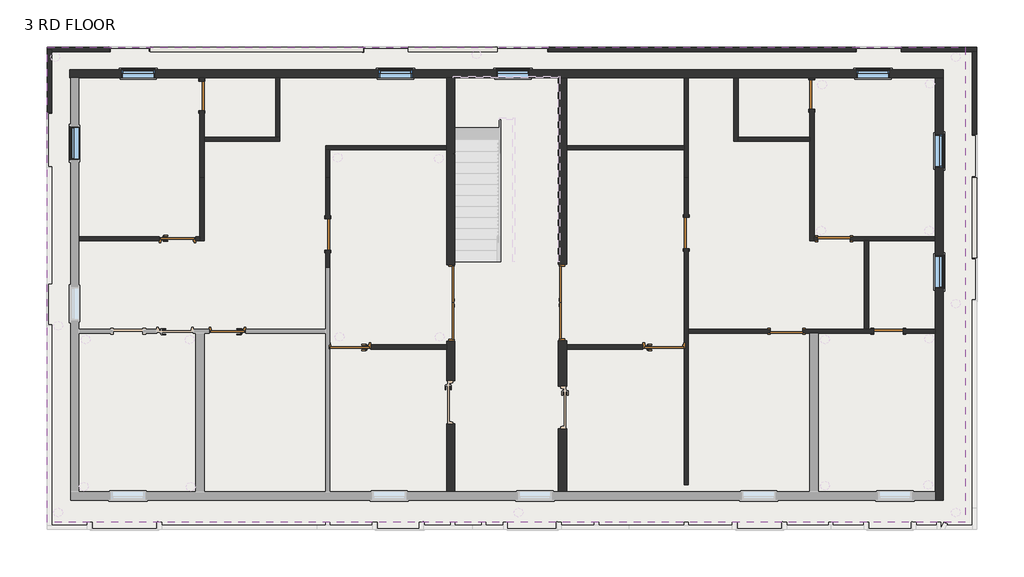
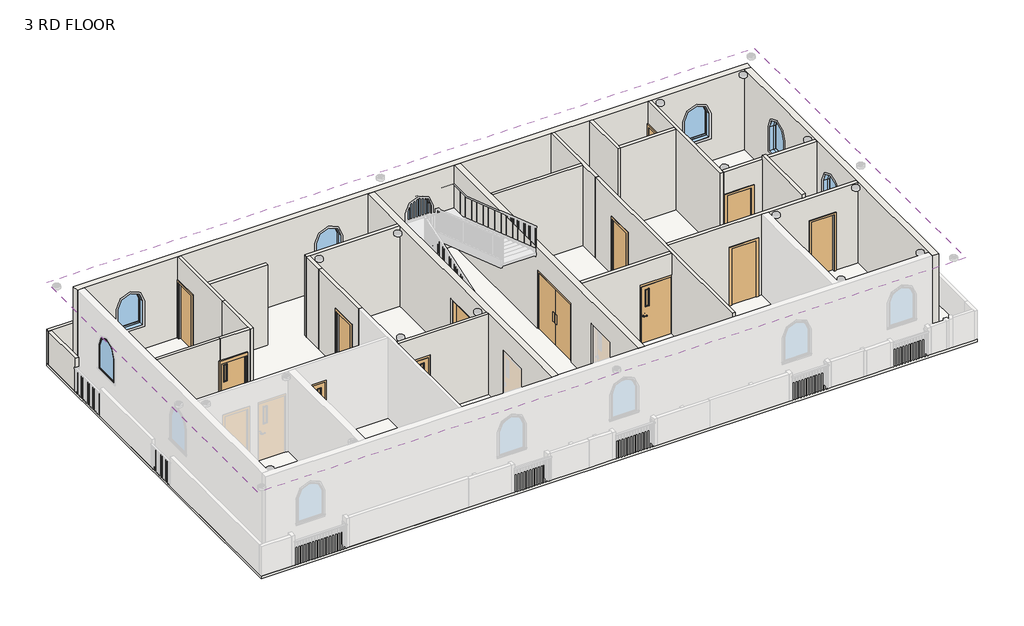
# One storey, part 2 of 7: 33 walls, 13 doors, 7 windows, 1 covering, 1 slab.
"""IFC4 building model written with IfcOpenShell, lengths in millimetres."""

from ifc_helpers import new_model, si_unit, frame, origin, place, context, project, spatial, polyline, circle_curve, outline, extrude, faceted_brep, transform, mapped, element, save
from ifc_brep_helpers import plane_surface, revolved_surface, advanced_brep
from components import door_2c854dd0, door_cf1f2706, door_4f5842df, door_passage_single_vision_lite_3_x7_440dd290, door_70e57c00, door_700d3439, door_8cb1b8a7, door_38851409, door_d141acb4, window_fixed_round_top_3_x_4_dee2be1c

model = new_model("IFC4")

# Units and contexts
model_context = context("Model", 3, world=origin())
ifc_project = project(units=[si_unit("LENGTHUNIT", "METRE", prefix="MILLI")], contexts=[model_context])

# Site, building, storey
site = spatial("IfcSite", under=ifc_project)
building = spatial("IfcBuilding", under=site)
storey = spatial("IfcBuildingStorey", under=building, Name="3 RD FLOOR", Elevation=9601.2)

# Covering
placement = place(None, origin())
element("IfcCovering", 1, ObjectType="2' x 4' ACT System", at=placement, inside=storey, context=model_context, shape_type="SweptSolid", body=[
    extrude(outline(polyline([(12235.5012075, 8470.0067329), (12235.5012075, -4623.6932193), (-13088.8067989, -4623.6932193), (-13088.8067989, 8470.0067329), (12235.5012075, 8470.0067329)])), frame((0.0, 0.0, 12649.2), z_axis=(0.0, 0.0, 1.0), x_axis=(1.0, 0.0, 0.0)), (0.0, 0.0, 1.0), 57.15),
])

# Doors
door_shape = door_2c854dd0(model_context)
element("IfcDoor", 2, ObjectType="Door-Passage-Double-Flush-Dbl_Acting : 6'79\" X 84\"", at=placement, inside=storey, context=model_context, shape_type="MappedRepresentation", body=[
    mapped(door_shape, transform((-1969.4487998, 1424.4578621, 9601.2), x_axis=(0.0, -1.0, 0.0), y_axis=(1.0, 0.0, 0.0), z_axis=(0.0, 0.0, 1.0))),
])
element("IfcDoor", 3, ObjectType="Door-Passage-Double-Flush-Dbl_Acting : 6'79\" X 84\"", at=placement, inside=storey, context=model_context, shape_type="MappedRepresentation", body=[
    mapped(door_shape, transform((1128.8432011, 1434.2067807, 9601.2), x_axis=(0.0, 1.0, 0.0), y_axis=(-1.0, 0.0, 0.0), z_axis=(0.0, 0.0, 1.0))),
])
door_2_shape = door_cf1f2706(model_context)
element("IfcDoor", 4, ObjectType="Door-Passage-Single-Vision_Lite : 3'6\"X7' 2", at=placement, inside=storey, context=model_context, shape_type="MappedRepresentation", body=[
    mapped(door_2_shape, transform((-4750.7487995, 211.6078621, 9601.2), x_axis=(-1.0, 0.0, 0.0), y_axis=(0.0, -1.0, 0.0), z_axis=(0.0, 0.0, 1.0))),
])
door_3_shape = door_4f5842df(model_context)
element("IfcDoor", 5, ObjectType="Door-Passage-Single-Vision_Lite : 3'6\"X7' 2", at=placement, inside=storey, context=model_context, shape_type="MappedRepresentation", body=[
    mapped(door_3_shape, transform((3923.3512082, 211.6078621, 9601.2), x_axis=(1.0, 0.0, 0.0), y_axis=(0.0, 1.0, 0.0), z_axis=(0.0, 0.0, 1.0))),
])
door_passage_single_vision_lite_3_x7_shape = door_passage_single_vision_lite_3_x7_440dd290(model_context)
element("IfcDoor", 6, ObjectType="Door-Passage-Single-Vision_Lite : 3'X7'", at=placement, inside=storey, context=model_context, shape_type="MappedRepresentation", body=[
    mapped(door_passage_single_vision_lite_3_x7_shape, transform((-9501.8462614, 3186.8067332, 9601.2), x_axis=(1.0, 0.0, 0.0), y_axis=(0.0, 1.0, 0.0), z_axis=(0.0, 0.0, 1.0))),
])
element("IfcDoor", 7, ObjectType="Door-Passage-Single-Vision_Lite : 3'X7'", at=placement, inside=storey, context=model_context, shape_type="MappedRepresentation", body=[
    mapped(door_passage_single_vision_lite_3_x7_shape, transform((-8122.5987992, 646.8067334, 9601.2), x_axis=(-1.0, 0.0, 0.0), y_axis=(0.0, -1.0, 0.0), z_axis=(0.0, 0.0, 1.0))),
])
door_4_shape = door_70e57c00(model_context)
element("IfcDoor", 8, ObjectType="Single-Flush : 2'10\" x 7'", at=placement, inside=storey, context=model_context, shape_type="MappedRepresentation", body=[
    mapped(door_4_shape, transform((-5360.3487995, 3313.8067802, 9601.2), x_axis=(0.0, -1.0, 0.0), y_axis=(1.0, 0.0, 0.0), z_axis=(0.0, 0.0, 1.0))),
])
door_5_shape = door_700d3439(model_context)
element("IfcDoor", 9, ObjectType="Single-Flush : 2'10\" x 7'", at=placement, inside=storey, context=model_context, shape_type="MappedRepresentation", body=[
    mapped(door_5_shape, transform((4532.9512082, 3351.906733, 9601.2), x_axis=(0.0, -1.0, 0.0), y_axis=(1.0, 0.0, 0.0), z_axis=(0.0, 0.0, 1.0))),
])
door_6_shape = door_8cb1b8a7(model_context)
element("IfcDoor", 10, ObjectType="Single-Flush : 2'11\"x 7'", at=placement, inside=storey, context=model_context, shape_type="MappedRepresentation", body=[
    mapped(door_6_shape, transform((8609.6512079, 3193.1567332, 9601.2), x_axis=(-1.0, 0.0, 0.0), y_axis=(0.0, -1.0, 0.0), z_axis=(0.0, 0.0, 1.0))),
])
element("IfcDoor", 11, ObjectType="Single-Flush : 2'11\"x 7'", at=placement, inside=storey, context=model_context, shape_type="MappedRepresentation", body=[
    mapped(door_6_shape, transform((7295.2012079, 640.4567334, 9601.2), x_axis=(1.0, 0.0, 0.0), y_axis=(0.0, 1.0, 0.0), z_axis=(0.0, 0.0, 1.0))),
])
door_7_shape = door_38851409(model_context)
element("IfcDoor", 12, ObjectType="Single-Flush : 2'8\"x 7'", at=placement, inside=storey, context=model_context, shape_type="MappedRepresentation", body=[
    mapped(door_7_shape, transform((-8827.4487992, 7136.5067329, 9601.2), x_axis=(0.0, 1.0, 0.0), y_axis=(-1.0, 0.0, 0.0), z_axis=(0.0, 0.0, 1.0))),
])
element("IfcDoor", 13, ObjectType="Single-Flush : 2'8\"x 7'", at=placement, inside=storey, context=model_context, shape_type="MappedRepresentation", body=[
    mapped(door_7_shape, transform((10111.5098918, 640.4567334, 9601.2), x_axis=(-1.0, 0.0, 0.0), y_axis=(0.0, -1.0, 0.0), z_axis=(0.0, 0.0, 1.0))),
])
door_8_shape = door_d141acb4(model_context)
element("IfcDoor", 14, ObjectType="Single-Flush : 2'8\"x 7'", at=placement, inside=storey, context=model_context, shape_type="MappedRepresentation", body=[
    mapped(door_8_shape, transform((8000.0512079, 7167.840939, 9601.2), x_axis=(0.0, 1.0, 0.0), y_axis=(-1.0, 0.0, 0.0), z_axis=(0.0, 0.0, 1.0))),
])

# Slab
element("IfcSlab", 15, ObjectType="LW Concrete on Metal Deck", at=placement, inside=storey, context=model_context, shape_type="SweptSolid", body=[
    extrude(outline(polyline([(12540.3012043, 8470.0067329), (12540.3012043, -4826.8932661), (-13088.8067989, -4826.8932661), (-13088.8067989, 8470.0067329), (12540.3012043, 8470.0067329)])), frame((0.0, 0.0, 9496.425), z_axis=(0.0, 0.0, 1.0), x_axis=(1.0, 0.0, 0.0)), (0.0, 0.0, 1.0), 104.775),
])

# Walls
element("IfcWall", 16, ObjectType="Generic - 4.5\"", at=placement, inside=storey, context=model_context, shape_type="SweptSolid", body=[
    extrude(outline(polyline([(12649.2, -9959.0462614), (12649.2, -12224.6987925), (9601.2, -12224.6987925), (9601.2, -10009.8462614), (11836.4, -10009.8462614), (11836.4, -9959.0462614), (12649.2, -9959.0462614)])), frame((0.0, 3136.0067332, 0.0), z_axis=(0.0, 1.0, 0.0), x_axis=(0.0, 0.0, 1.0)), (0.0, 0.0, 1.0), 114.3),
])
element("IfcWall", 17, ObjectType="Generic - 4.5\"", at=placement, inside=storey, context=model_context, shape_type="Brep", body=[
    faceted_brep([(-8884.5987992, 4875.906733, 9601.2), (-8884.5987992, 3250.3067332, 9601.2), (-8884.5987992, 3136.0067332, 9601.2), (-8884.5987992, 3136.0067332, 12649.2), (-8884.5987992, 3250.3067332, 12649.2), (-8884.5987992, 4875.906733, 12649.2), (-8770.2987992, 4875.906733, 9601.2), (-8770.2987992, 4875.906733, 12649.2), (-8770.2987992, 3136.0067332, 12649.2), (-8770.2987992, 3136.0067332, 9601.2)], [[[0, 1, 2, 3, 4, 5]], [[6, 7, 8, 9]], [[2, 1, 0, 6, 9]], [[5, 4, 3, 8, 7]], [[0, 5, 7, 6]], [[3, 2, 9, 8]]]),
])
element("IfcWall", 18, ObjectType="Generic - 4.5\"", at=placement, inside=storey, context=model_context, shape_type="SweptSolid", body=[
    extrude(outline(polyline([(12649.2, -2077.3987998), (12649.2, -5303.1987995), (11836.4, -5303.1987995), (11836.4, -4166.5487995), (9601.2, -4166.5487995), (9601.2, -2077.3987998), (12649.2, -2077.3987998)])), frame((0.0, 148.1078621, 0.0), z_axis=(0.0, 1.0, 0.0), x_axis=(0.0, 0.0, 1.0)), (0.0, 0.0, 1.0), 114.3),
])
element("IfcWall", 19, ObjectType="Generic - 4.5\"", at=placement, inside=storey, context=model_context, shape_type="Brep", body=[
    faceted_brep([(-2077.3987998, 5764.9067329, 9601.2), (-5417.4987995, 5764.9067329, 9601.2), (-5417.4987995, 5764.9067329, 12649.2), (-2077.3987998, 5764.9067329, 12649.2), (-2077.3987998, 5650.6067329, 9601.2), (-2077.3987998, 5650.6067329, 12649.2), (-5303.1987995, 5650.6067329, 12649.2), (-5417.4987995, 5650.6067329, 12649.2), (-5417.4987995, 5650.6067329, 9601.2), (-5303.1987995, 5650.6067329, 9601.2)], [[[0, 1, 2, 3]], [[4, 5, 6, 7, 8, 9]], [[1, 0, 4, 9, 8]], [[3, 2, 7, 6, 5]], [[2, 1, 8, 7]], [[0, 3, 5, 4]]]),
])
element("IfcWall", 20, ObjectType="Generic - 4.5\"", at=placement, inside=storey, context=model_context, shape_type="SweptSolid", body=[
    extrude(outline(polyline([(-5417.4987995, 4875.90678), (-5417.4987995, 5650.6067329), (-5303.1987995, 5650.6067329), (-5303.1987995, 4875.90678), (-5417.4987995, 4875.90678)])), frame((0.0, 0.0, 9601.2), z_axis=(0.0, 0.0, 1.0), x_axis=(1.0, 0.0, 0.0)), (0.0, 0.0, 1.0), 3048.0),
])
element("IfcWall", 21, ObjectType="Generic - 4.5\"", at=placement, inside=storey, context=model_context, shape_type="SweptSolid", body=[
    extrude(outline(polyline([(4475.8012082, 5650.6067329), (1250.0012085, 5650.6067329), (1250.0012085, 5764.9067329), (4475.8012082, 5764.9067329), (4475.8012082, 5650.6067329)])), frame((0.0, 0.0, 9601.2), z_axis=(0.0, 0.0, 1.0), x_axis=(1.0, 0.0, 0.0)), (0.0, 0.0, 1.0), 3048.0),
])
element("IfcWall", 22, ObjectType="Generic - 4.5\"", at=placement, inside=storey, context=model_context, shape_type="Brep", body=[
    faceted_brep([(4475.8012082, 7631.8067329, 9601.2), (4475.8012082, 5764.9067329, 9601.2), (4475.8012082, 5650.6067329, 9601.2), (4475.8012082, 4875.906733, 9601.2), (4475.8012082, 4875.906733, 12649.2), (4475.8012082, 5650.6067329, 12649.2), (4475.8012082, 5764.9067329, 12649.2), (4475.8012082, 7631.8067329, 12649.2), (4590.1012082, 7631.8067329, 9601.2), (4590.1012082, 7631.8067329, 12649.2), (4590.1012082, 4875.906733, 12649.2), (4590.1012082, 4875.906733, 9601.2)], [[[0, 1, 2, 3, 4, 5, 6, 7]], [[8, 9, 10, 11]], [[3, 2, 1, 0, 8, 11]], [[4, 3, 11, 10]], [[7, 6, 5, 4, 10, 9]], [[0, 7, 9, 8]]]),
])
element("IfcWall", 23, ObjectType="Generic - 4.5\"", at=placement, inside=storey, context=model_context, shape_type="Brep", body=[
    faceted_brep([(4475.8012082, -3594.9932193, 9601.2), (4475.8012082, -3594.9932193, 12649.2), (4475.8012082, 148.1078621, 12649.2), (4475.8012082, 262.4078621, 12649.2), (4475.8012082, 4875.906733, 12649.2), (4475.8012082, 4875.906733, 9601.2), (4475.8012082, 3783.706733, 9601.2), (4475.8012082, 3783.706733, 11734.8), (4475.8012082, 2920.106733, 11734.8), (4475.8012082, 2920.106733, 9601.2), (4475.8012082, 262.4078621, 9601.2), (4475.8012082, 262.4078621, 11836.4), (4475.8012082, 148.1078621, 11836.4), (4475.8012082, 148.1078621, 9601.2), (4590.1012082, -3594.9932193, 12649.2), (4590.1012082, -3594.9932193, 9601.2), (4590.1012082, 583.3067334, 9601.2), (4590.1012082, 697.6067334, 9601.2), (4590.1012082, 2920.106733, 9601.2), (4590.1012082, 2920.106733, 11734.8), (4590.1012082, 3783.706733, 11734.8), (4590.1012082, 3783.706733, 9601.2), (4590.1012082, 4875.906733, 9601.2), (4590.1012082, 4875.906733, 12649.2), (4590.1012082, 697.6067334, 12649.2), (4590.1012082, 583.3067334, 12649.2), (4507.5512082, 148.1078621, 9601.2), (4507.5512082, 262.4078621, 9601.2), (4507.5512082, 148.1078621, 11836.4), (4507.5512082, 262.4078621, 11836.4)], [[[0, 1, 2, 3, 4, 5, 6, 7, 8, 9, 10, 11, 12, 13]], [[14, 15, 16, 17, 18, 19, 20, 21, 22, 23, 24, 25]], [[15, 0, 13, 26, 27, 10, 9, 18, 17, 16]], [[5, 22, 21, 6]], [[1, 0, 15, 14]], [[4, 3, 2, 1, 14, 25, 24, 23]], [[5, 4, 23, 22]], [[19, 18, 9, 8]], [[20, 19, 8, 7]], [[21, 20, 7, 6]], [[28, 26, 13, 12]], [[27, 29, 11, 10]], [[26, 28, 29, 27]], [[29, 28, 12, 11]]]),
])
element("IfcWall", 24, ObjectType="Generic - 4.5\"", at=placement, inside=storey, context=model_context, shape_type="Brep", body=[
    faceted_brep([(5847.401208, 7631.8067329, 9601.2), (5847.401208, 5879.2067329, 9601.2), (5847.401208, 5879.2067329, 12649.2), (5847.401208, 7631.8067329, 12649.2), (5961.701208, 7631.8067329, 9601.2), (5961.701208, 7631.8067329, 12649.2), (5961.701208, 5993.5067329, 12649.2), (5961.701208, 5879.2067329, 12649.2), (5961.701208, 5879.2067329, 9601.2), (5961.701208, 5993.5067329, 9601.2)], [[[0, 1, 2, 3]], [[4, 5, 6, 7, 8, 9]], [[1, 0, 4, 9, 8]], [[3, 2, 7, 6, 5]], [[0, 3, 5, 4]], [[2, 1, 8, 7]]]),
])
element("IfcWall", 25, ObjectType="Generic - 4.5\"", at=placement, inside=storey, context=model_context, shape_type="SweptSolid", body=[
    extrude(outline(polyline([(7942.9012079, 5879.2067329), (5961.701208, 5879.2067329), (5961.701208, 5993.5067329), (7942.9012079, 5993.5067329), (7942.9012079, 5879.2067329)])), frame((0.0, 0.0, 9601.2), z_axis=(0.0, 0.0, 1.0), x_axis=(1.0, 0.0, 0.0)), (0.0, 0.0, 1.0), 3048.0),
])
element("IfcWall", 26, ObjectType="Generic - 4.5\"", at=placement, inside=storey, context=model_context, shape_type="Brep", body=[
    faceted_brep([(7942.9012079, 7625.040939, 9601.2), (7942.9012079, 7574.240939, 9601.2), (7942.9012079, 7574.240939, 11734.8), (7942.9012079, 6761.440939, 11734.8), (7942.9012079, 6761.440939, 9601.2), (7942.9012079, 5993.5067329, 9601.2), (7942.9012079, 5879.2067329, 9601.2), (7942.9012079, 3136.0067332, 9601.2), (7942.9012079, 3136.0067332, 12649.2), (7942.9012079, 5879.2067329, 12649.2), (7942.9012079, 5993.5067329, 12649.2), (7942.9012079, 7625.040939, 12649.2), (8057.2012079, 7574.240939, 11734.8), (8057.2012079, 7574.240939, 9601.2), (8057.2012079, 7625.040939, 9601.2), (8057.2012079, 7625.040939, 12649.2), (8057.2012079, 3250.3067332, 12649.2), (8057.2012079, 3136.0067332, 12649.2), (8057.2012079, 3136.0067332, 9601.2), (8057.2012079, 3250.3067332, 9601.2), (8057.2012079, 6761.440939, 9601.2), (8057.2012079, 6761.440939, 11734.8)], [[[0, 1, 2, 3, 4, 5, 6, 7, 8, 9, 10, 11]], [[12, 13, 14, 15, 16, 17, 18, 19, 20, 21]], [[14, 13, 1, 0]], [[20, 19, 18, 7, 6, 5, 4]], [[11, 10, 9, 8, 17, 16, 15]], [[0, 11, 15, 14]], [[8, 7, 18, 17]], [[2, 1, 13, 12]], [[3, 2, 12, 21]], [[4, 3, 21, 20]]]),
])
element("IfcWall", 27, ObjectType="Generic - 4.5\"", at=placement, inside=storey, context=model_context, shape_type="Brep", body=[
    faceted_brep([(8165.1512079, 3250.3067332, 11734.8), (8165.1512079, 3250.3067332, 9601.2), (8057.2012079, 3250.3067332, 9601.2), (8057.2012079, 3250.3067332, 12649.2), (11397.3012075, 3250.3067332, 12649.2), (11397.3012075, 3250.3067332, 9601.2), (9054.1512079, 3250.3067332, 9601.2), (9054.1512079, 3250.3067332, 11734.8), (8057.2012079, 3136.0067332, 9601.2), (8165.1512079, 3136.0067332, 9601.2), (8165.1512079, 3136.0067332, 11734.8), (9054.1512079, 3136.0067332, 11734.8), (9054.1512079, 3136.0067332, 9601.2), (9438.4098918, 3136.0067332, 9601.2), (9565.4098918, 3136.0067332, 9601.2), (11397.3012075, 3136.0067332, 9601.2), (11397.3012075, 3136.0067332, 12649.2), (8057.2012079, 3136.0067332, 12649.2)], [[[0, 1, 2, 3, 4, 5, 6, 7]], [[8, 9, 10, 11, 12, 13, 14, 15, 16, 17]], [[6, 5, 15, 14, 13, 12]], [[2, 1, 9, 8]], [[4, 3, 17, 16]], [[3, 2, 8, 17]], [[5, 4, 16, 15]], [[10, 9, 1, 0]], [[11, 10, 0, 7]], [[12, 11, 7, 6]]]),
])
element("IfcWall", 28, ObjectType="Generic - 4.5\"", at=placement, inside=storey, context=model_context, shape_type="Brep", body=[
    faceted_brep([(7739.7012079, 583.3067334, 11734.8), (7739.7012079, 583.3067334, 9601.2), (7942.9012079, 583.3067334, 9601.2), (8171.5012079, 583.3067334, 9601.2), (9705.1098918, 583.3067334, 9601.2), (9705.1098918, 583.3067334, 11734.8), (10517.9098918, 583.3067334, 11734.8), (10517.9098918, 583.3067334, 9601.2), (11397.3012075, 583.3067334, 9601.2), (11397.3012075, 583.3067334, 12649.2), (8171.5012079, 583.3067334, 12649.2), (7942.9012079, 583.3067334, 12649.2), (4590.1012082, 583.3067334, 12649.2), (4590.1012082, 583.3067334, 9601.2), (6850.7012079, 583.3067334, 9601.2), (6850.7012079, 583.3067334, 11734.8), (9705.1098918, 697.6067334, 9601.2), (9565.4098918, 697.6067334, 9601.2), (9438.4098918, 697.6067334, 9601.2), (7739.7012079, 697.6067334, 9601.2), (7739.7012079, 697.6067334, 11734.8), (6850.7012079, 697.6067334, 11734.8), (6850.7012079, 697.6067334, 9601.2), (4590.1012082, 697.6067334, 9601.2), (4590.1012082, 697.6067334, 12649.2), (11397.3012075, 697.6067334, 12649.2), (11397.3012075, 697.6067334, 9601.2), (10517.9098918, 697.6067334, 9601.2), (10517.9098918, 697.6067334, 11734.8), (9705.1098918, 697.6067334, 11734.8)], [[[0, 1, 2, 3, 4, 5, 6, 7, 8, 9, 10, 11, 12, 13, 14, 15]], [[16, 17, 18, 19, 20, 21, 22, 23, 24, 25, 26, 27, 28, 29]], [[27, 26, 8, 7]], [[14, 13, 23, 22]], [[4, 3, 2, 1, 19, 18, 17, 16]], [[12, 11, 10, 9, 25, 24]], [[9, 8, 26, 25]], [[13, 12, 24, 23]], [[5, 4, 16, 29]], [[6, 5, 29, 28]], [[7, 6, 28, 27]], [[20, 19, 1, 0]], [[21, 20, 0, 15]], [[22, 21, 15, 14]]]),
])
element("IfcWall", 29, ObjectType="Generic - 4.5\"", at=placement, inside=storey, context=model_context, shape_type="Brep", body=[
    faceted_brep([(-8770.2987992, 7542.9067329, 11734.8), (-8770.2987992, 7542.9067329, 9601.2), (-8770.2987992, 7631.8067329, 9601.2), (-8770.2987992, 7631.8067329, 12649.2), (-8770.2987992, 5993.5067329, 12649.2), (-8770.2987992, 5879.2067329, 12649.2), (-8770.2987992, 4875.906733, 12649.2), (-8770.2987992, 4875.906733, 9601.2), (-8770.2987992, 5879.2067329, 9601.2), (-8770.2987992, 5993.5067329, 9601.2), (-8770.2987992, 6730.1067329, 9601.2), (-8770.2987992, 6730.1067329, 11734.8), (-8884.5987992, 7631.8067329, 9601.2), (-8884.5987992, 7542.9067329, 9601.2), (-8884.5987992, 7542.9067329, 11734.8), (-8884.5987992, 6730.1067329, 11734.8), (-8884.5987992, 6730.1067329, 9601.2), (-8884.5987992, 4875.906733, 9601.2), (-8884.5987992, 4875.906733, 12649.2), (-8884.5987992, 7631.8067329, 12649.2)], [[[0, 1, 2, 3, 4, 5, 6, 7, 8, 9, 10, 11]], [[12, 13, 14, 15, 16, 17, 18, 19]], [[2, 1, 13, 12]], [[10, 9, 8, 7, 17, 16]], [[6, 5, 4, 3, 19, 18]], [[7, 6, 18, 17]], [[3, 2, 12, 19]], [[14, 13, 1, 0]], [[15, 14, 0, 11]], [[16, 15, 11, 10]]]),
])
element("IfcWall", 30, ObjectType="Generic - 4.5\"", at=placement, inside=storey, context=model_context, shape_type="Brep", body=[
    faceted_brep([(-8770.2987992, 5879.2067329, 9601.2), (-6674.7987994, 5879.2067329, 9601.2), (-6674.7987994, 5879.2067329, 12649.2), (-8770.2987992, 5879.2067329, 12649.2), (-8770.2987992, 5993.5067329, 9601.2), (-8770.2987992, 5993.5067329, 12649.2), (-6674.7987994, 5993.5067329, 12649.2), (-6674.7987994, 5993.5067329, 10972.8), (-6674.7987994, 5993.5067329, 9601.2), (-6789.0987994, 5993.5067329, 9601.2)], [[[0, 1, 2, 3]], [[4, 5, 6, 7, 8, 9]], [[1, 0, 4, 9, 8]], [[3, 2, 6, 5]], [[0, 3, 5, 4]], [[2, 1, 8, 7, 6]]]),
])
element("IfcWall", 31, ObjectType="Generic - 4.5\"", at=placement, inside=storey, context=model_context, shape_type="SweptSolid", body=[
    extrude(outline(polyline([(-6674.7987994, 7631.8067329), (-6674.7987994, 5993.5067329), (-6789.0987994, 5993.5067329), (-6789.0987994, 7631.8067329), (-6674.7987994, 7631.8067329)])), frame((0.0, 0.0, 9601.2), z_axis=(0.0, 0.0, 1.0), x_axis=(1.0, 0.0, 0.0)), (0.0, 0.0, 1.0), 1371.6),
])
element("IfcWall", 32, ObjectType="Generic - 4.5\"", at=placement, inside=storey, context=model_context, shape_type="SweptSolid", body=[
    extrude(outline(polyline([(12649.2, -8884.5987992), (12649.2, -9959.0462614), (11836.4, -9959.0462614), (11836.4, -8993.8462614), (9601.2, -8993.8462614), (9601.2, -8884.5987992), (12649.2, -8884.5987992)])), frame((0.0, 3136.0067332, 0.0), z_axis=(0.0, 1.0, 0.0), x_axis=(0.0, 0.0, 1.0)), (0.0, 0.0, 1.0), 114.3),
])
element("IfcWall", 33, ObjectType="Generic - 4.5\"", at=placement, inside=storey, context=model_context, shape_type="SweptSolid", body=[
    extrude(outline(polyline([(2882.0067802, 11734.8), (2882.0067802, 9601.2), (2399.4067802, 9601.2), (2399.4067802, 12649.2), (4875.90678, 12649.2), (4875.90678, 9601.2), (3745.6067802, 9601.2), (3745.6067802, 11734.8), (2882.0067802, 11734.8)])), frame((-5417.4987995, 0.0, 0.0), z_axis=(1.0, 0.0, 0.0), x_axis=(0.0, 1.0, 0.0)), (0.0, 0.0, 1.0), 114.3),
])
element("IfcWall", 34, ObjectType="Generic - 4.5\"", at=placement, inside=storey, context=model_context, shape_type="SweptSolid", body=[
    extrude(outline(polyline([(12649.2, 4475.8012082), (12649.2, 1250.0012085), (9601.2, 1250.0012085), (9601.2, 3339.1512082), (11836.4, 3339.1512082), (11836.4, 4475.8012082), (12649.2, 4475.8012082)])), frame((0.0, 148.1078621, 0.0), z_axis=(0.0, 1.0, 0.0), x_axis=(0.0, 0.0, 1.0)), (0.0, 0.0, 1.0), 114.3),
])
element("IfcWall", 35, ObjectType="Generic - 4.5\"", at=placement, inside=storey, context=model_context, shape_type="SweptSolid", body=[
    extrude(outline(polyline([(-12973.9987925, 8412.8567329), (-12973.9987925, 6682.2711337), (-13088.2987925, 6682.2711337), (-13088.2987925, 8412.8567329), (-12973.9987925, 8412.8567329)])), frame((0.0, 0.0, 9601.2), z_axis=(0.0, 0.0, 1.0), x_axis=(1.0, 0.0, 0.0)), (0.0, 0.0, 1.0), 1259.0059812),
])
element("IfcWall", 36, ObjectType="Generic - 4.5\"", at=placement, inside=storey, context=model_context, shape_type="SweptSolid", body=[
    extrude(outline(polyline([(-11387.0067989, 8355.7067329), (-13088.8067989, 8355.7067329), (-13088.8067989, 8470.0067329), (-11387.0067989, 8470.0067329), (-11387.0067989, 8355.7067329)])), frame((0.0, 0.0, 9601.2), z_axis=(0.0, 0.0, 1.0), x_axis=(1.0, 0.0, 0.0)), (0.0, 0.0, 1.0), 1273.4134002),
])
element("IfcWall", 37, ObjectType="Generic - 4.5\"", at=placement, inside=storey, context=model_context, shape_type="SweptSolid", body=[
    extrude(outline(polyline([(-4382.4487992, 8355.7067329), (-10247.1817989, 8355.7067329), (-10247.1817989, 8470.0067329), (-4382.4487992, 8470.0067329), (-4382.4487992, 8355.7067329)])), frame((0.0, 0.0, 9601.2), z_axis=(0.0, 0.0, 1.0), x_axis=(1.0, 0.0, 0.0)), (0.0, 0.0, 1.0), 1083.89837),
])
element("IfcWall", 38, ObjectType="Generic - 4.5\"", at=placement, inside=storey, context=model_context, shape_type="SweptSolid", body=[
    extrude(outline(polyline([(-682.0490672, 8355.7067329), (-3139.4990672, 8355.7067329), (-3139.4990672, 8470.0067329), (-682.0490672, 8470.0067329), (-682.0490672, 8355.7067329)])), frame((0.0, 0.0, 9601.2), z_axis=(0.0, 0.0, 1.0), x_axis=(1.0, 0.0, 0.0)), (0.0, 0.0, 1.0), 1195.9732529),
])
element("IfcWall", 39, ObjectType="Generic - 4.5\"", at=placement, inside=storey, context=model_context, shape_type="SweptSolid", body=[
    extrude(outline(polyline([(9199.6932011, 8355.7067329), (741.4932011, 8355.7067329), (741.4932011, 8470.0067329), (9199.6932011, 8470.0067329), (9199.6932011, 8355.7067329)])), frame((0.0, 0.0, 9601.2), z_axis=(0.0, 0.0, 1.0), x_axis=(1.0, 0.0, 0.0)), (0.0, 0.0, 1.0), 1274.1868366),
])
element("IfcWall", 40, ObjectType="Generic - 4.5\"", at=placement, inside=storey, context=model_context, shape_type="Brep", body=[
    faceted_brep([(10462.2009401, 8355.7067329, 9601.2), (12426.0012043, 8355.7067329, 9601.2), (12540.3012043, 8355.7067329, 9601.2), (12540.3012043, 8355.7067329, 10966.9502881), (10462.2009401, 8355.7067329, 10966.9502881), (10462.2009401, 8470.0067329, 9601.2), (10462.2009401, 8470.0067329, 10966.9502881), (12540.3012043, 8470.0067329, 10966.9502881), (12540.3012043, 8470.0067329, 9601.2)], [[[0, 1, 2, 3, 4]], [[5, 6, 7, 8]], [[2, 1, 0, 5, 8]], [[4, 3, 7, 6]], [[0, 4, 6, 5]], [[3, 2, 8, 7]]]),
])
element("IfcWall", 41, ObjectType="Generic - 4.5\"", at=placement, inside=storey, context=model_context, shape_type="Brep", body=[
    faceted_brep([(12426.0012043, 8355.7067329, 9601.2), (12426.0012043, 6069.7067329, 9601.2), (12426.0012043, 6069.7067329, 10972.8), (12426.0012043, 8355.7067329, 10972.8), (12540.3012043, 8355.7067329, 9601.2), (12540.3012043, 8355.7067329, 10966.9502881), (12540.3012043, 8355.7067329, 10972.8), (12540.3012043, 6069.7067329, 10972.8), (12540.3012043, 6069.7067329, 9601.2)], [[[0, 1, 2, 3]], [[4, 5, 6, 7, 8]], [[1, 0, 4, 8]], [[2, 1, 8, 7]], [[3, 2, 7, 6]], [[0, 3, 6, 5, 4]]]),
])
element("IfcWall", 42, ObjectType="Generic - 4.5\"", at=placement, inside=storey, context=model_context, shape_type="SweptSolid", body=[
    extrude(outline(polyline([(12426.0012043, 2666.1067329), (12426.0012043, 4875.9067329), (12540.3012043, 4875.9067329), (12540.3012043, 2666.1067329), (12426.0012043, 2666.1067329)])), frame((0.0, 0.0, 9601.2), z_axis=(0.0, 0.0, 1.0), x_axis=(1.0, 0.0, 0.0)), (0.0, 0.0, 1.0), 1193.0409005),
])
element("IfcWall", 43, ObjectType="Generic - 9\"", at=placement, inside=storey, context=model_context, shape_type="AdvancedBrep", body=[
    advanced_brep(
    [(-12479.2067989, 7631.8067329, 9601.2), (-12453.2987925, 7631.8067329, 9601.2), (-12224.6987925, 7631.8067329, 9601.2), (-8884.5987992, 7631.8067329, 9601.2), (-8770.2987992, 7631.8067329, 9601.2), (-6789.0987994, 7631.8067329, 9601.2), (-6674.7987994, 7631.8067329, 9601.2), (-2077.3987998, 7631.8067329, 9601.2), (-1848.7987998, 7631.8067329, 9601.2), (1008.1932011, 7631.8067329, 9601.2), (1236.7932011, 7631.8067329, 9601.2), (4475.8012082, 7631.8067329, 9601.2), (4590.1012082, 7631.8067329, 9601.2), (5847.401208, 7631.8067329, 9601.2), (5961.701208, 7631.8067329, 9601.2), (11397.3012075, 7631.8067329, 9601.2), (11625.9012075, 7631.8067329, 9601.2), (11625.9012075, 7631.8067329, 12649.2), (11397.3012075, 7631.8067329, 12649.2), (5961.701208, 7631.8067329, 12649.2), (5847.401208, 7631.8067329, 12649.2), (4590.1012082, 7631.8067329, 12649.2), (4475.8012082, 7631.8067329, 12649.2), (1236.7932011, 7631.8067329, 12649.2), (1008.1932011, 7631.8067329, 12649.2), (-1848.7987998, 7631.8067329, 12649.2), (-2077.3987998, 7631.8067329, 12649.2), (-8770.2987992, 7631.8067329, 12649.2), (-8884.5987992, 7631.8067329, 12649.2), (-12224.6987925, 7631.8067329, 12649.2), (-12453.2987925, 7631.8067329, 12649.2), (-12479.2067989, 7631.8067329, 12649.2), (9225.6012075, 7631.8067329, 10515.6), (9225.6012075, 7631.8067329, 11430.0), (10140.0012075, 7631.8067329, 11430.0), (10140.0012075, 7631.8067329, 10515.6), (-706.3067989, 7631.8067329, 10515.6), (-706.3067989, 7631.8067329, 11430.0), (208.0932011, 7631.8067329, 11430.0), (208.0932011, 7631.8067329, 10515.6), (-3944.2987998, 7631.8067329, 10515.6), (-3944.2987998, 7631.8067329, 11430.0), (-3029.8987998, 7631.8067329, 11430.0), (-3029.8987998, 7631.8067329, 10515.6), (-11040.4237959, 7631.8067329, 10515.6), (-11040.4237959, 7631.8067329, 11430.0), (-10126.0237959, 7631.8067329, 11430.0), (-10126.0237959, 7631.8067329, 10515.6), (-12479.2067989, 7860.4067329, 9601.2), (-12479.2067989, 7860.4067329, 12649.2), (11625.9012075, 7860.4067329, 12649.2), (11625.9012075, 7860.4067329, 9601.2), (9225.6012075, 7860.4067329, 10515.6), (10140.0012075, 7860.4067329, 10515.6), (10140.0012075, 7860.4067329, 11430.0), (9225.6012075, 7860.4067329, 11430.0), (-706.3067989, 7860.4067329, 10515.6), (208.0932011, 7860.4067329, 10515.6), (208.0932011, 7860.4067329, 11430.0), (-706.3067989, 7860.4067329, 11430.0), (-3944.2987998, 7860.4067329, 10515.6), (-3029.8987998, 7860.4067329, 10515.6), (-3029.8987998, 7860.4067329, 11430.0), (-3944.2987998, 7860.4067329, 11430.0), (-11040.4237959, 7860.4067329, 10515.6), (-10126.0237959, 7860.4067329, 10515.6), (-10126.0237959, 7860.4067329, 11430.0), (-11040.4237959, 7860.4067329, 11430.0)],
    [
        (0, 1),
        (1, 2),
        (2, 3),
        (3, 4),
        (4, 5),
        (5, 6),
        (6, 7),
        (7, 8),
        (8, 9),
        (9, 10),
        (10, 11),
        (11, 12),
        (12, 13),
        (13, 14),
        (14, 15),
        (15, 16),
        (16, 17),
        (17, 18),
        (18, 19),
        (19, 20),
        (20, 21),
        (21, 22),
        (22, 23),
        (23, 24),
        (24, 25),
        (25, 26),
        (26, 27),
        (27, 28),
        (28, 29),
        (29, 30),
        (30, 31),
        (31, 0),
        (32, 33),
        (33, 34, circle_curve(frame((9682.8012075, 7631.8067329, 11430.0), z_axis=(0.0, 1.0, 0.0), x_axis=(1.0, 0.0, 0.0)), 457.2)),
        (34, 35),
        (35, 32),
        (36, 37),
        (37, 38, circle_curve(frame((-249.1067989, 7631.8067329, 11430.0), z_axis=(0.0, 1.0, 0.0), x_axis=(1.0, 0.0, 0.0)), 457.2)),
        (38, 39),
        (39, 36),
        (40, 41),
        (41, 42, circle_curve(frame((-3487.0987998, 7631.8067329, 11430.0), z_axis=(0.0, 1.0, 0.0), x_axis=(1.0, 0.0, 0.0)), 457.2)),
        (42, 43),
        (43, 40),
        (44, 45),
        (45, 46, circle_curve(frame((-10583.2237959, 7631.8067329, 11430.0), z_axis=(0.0, 1.0, 0.0), x_axis=(1.0, 0.0, 0.0)), 457.2)),
        (46, 47),
        (47, 44),
        (48, 49),
        (49, 50),
        (50, 51),
        (51, 48),
        (52, 53),
        (53, 54),
        (54, 55, circle_curve(frame((9682.8012075, 7860.4067329, 11430.0), z_axis=(0.0, -1.0, 0.0), x_axis=(1.0, 0.0, 0.0)), 457.2)),
        (55, 52),
        (56, 57),
        (57, 58),
        (58, 59, circle_curve(frame((-249.1067989, 7860.4067329, 11430.0), z_axis=(0.0, -1.0, 0.0), x_axis=(1.0, 0.0, 0.0)), 457.2)),
        (59, 56),
        (60, 61),
        (61, 62),
        (62, 63, circle_curve(frame((-3487.0987998, 7860.4067329, 11430.0), z_axis=(0.0, -1.0, 0.0), x_axis=(1.0, 0.0, 0.0)), 457.2)),
        (63, 60),
        (64, 65),
        (65, 66),
        (66, 67, circle_curve(frame((-10583.2237959, 7860.4067329, 11430.0), z_axis=(0.0, -1.0, 0.0), x_axis=(1.0, 0.0, 0.0)), 457.2)),
        (67, 64),
        (0, 48),
        (51, 16),
        (17, 50),
        (49, 31),
        (52, 32),
        (35, 53),
        (34, 54),
        (33, 55),
        (56, 36),
        (39, 57),
        (38, 58),
        (37, 59),
        (60, 40),
        (43, 61),
        (42, 62),
        (41, 63),
        (64, 44),
        (47, 65),
        (46, 66),
        (45, 67),
    ],
    [
        plane_surface(frame((-12479.2067989, 7631.8067329, 9601.2), z_axis=(0.0, -1.0, 0.0), x_axis=(1.0, 0.0, 0.0))),
        plane_surface(frame((-12479.2067989, 7860.4067329, 9601.2), z_axis=(0.0, 1.0, 0.0), x_axis=(-1.0, 0.0, 0.0))),
        plane_surface(frame((-12479.2067989, 7631.8067329, 9601.2), z_axis=(0.0, 0.0, -1.0), x_axis=(0.0, 1.0, 0.0))),
        plane_surface(frame((11511.6012075, 7631.8067329, 12649.2), z_axis=(0.0, 0.0, 1.0), x_axis=(0.0, 1.0, 0.0))),
        plane_surface(frame((-12479.2067989, 7631.8067329, 12649.2), z_axis=(-1.0, 0.0, 0.0), x_axis=(0.0, 1.0, 0.0))),
        plane_surface(frame((11625.9012075, 7629.6366753, 9601.2), z_axis=(1.0, 0.0, 0.0), x_axis=(0.0, 1.0, 0.0))),
        plane_surface(frame((9225.6012075, 7860.4067329, 10515.6), z_axis=(0.0, 0.0, 1.0), x_axis=(0.0, -1.0, 0.0))),
        plane_surface(frame((10140.0012075, 7860.4067329, 10515.6), z_axis=(-1.0, 0.0, 0.0), x_axis=(0.0, -1.0, 0.0))),
        revolved_surface(polyline([(10140.001207500001, 7631.8067329, 11430.0), (10140.001207500001, 7860.4067329, 11430.0)]), (9682.8012075, 7631.8067329, 11430.0), (0.0, -1.0, 0.0)),
        plane_surface(frame((9225.6012075, 7860.4067329, 11430.0), z_axis=(1.0, 0.0, 0.0), x_axis=(0.0, -1.0, 0.0))),
        plane_surface(frame((-706.3067989, 7860.4067329, 10515.6), z_axis=(0.0, 0.0, 1.0), x_axis=(0.0, -1.0, 0.0))),
        plane_surface(frame((208.0932011, 7860.4067329, 10515.6), z_axis=(-1.0, 0.0, 0.0), x_axis=(0.0, -1.0, 0.0))),
        revolved_surface(polyline([(208.0932011, 7631.8067329, 11430.0), (208.0932011, 7860.4067329, 11430.0)]), (-249.1067989, 7631.8067329, 11430.0), (0.0, -1.0, 0.0)),
        plane_surface(frame((-706.3067989, 7860.4067329, 11430.0), z_axis=(1.0, 0.0, 0.0), x_axis=(0.0, -1.0, 0.0))),
        plane_surface(frame((-3944.2987998, 7860.4067329, 10515.6), z_axis=(0.0, 0.0, 1.0), x_axis=(0.0, -1.0, 0.0))),
        plane_surface(frame((-3029.8987998, 7860.4067329, 10515.6), z_axis=(-1.0, 0.0, 0.0), x_axis=(0.0, -1.0, 0.0))),
        revolved_surface(polyline([(-3029.8987998000002, 7631.8067329, 11430.0), (-3029.8987998000002, 7860.4067329, 11430.0)]), (-3487.0987998, 7631.8067329, 11430.0), (0.0, -1.0, 0.0)),
        plane_surface(frame((-3944.2987998, 7860.4067329, 11430.0), z_axis=(1.0, 0.0, 0.0), x_axis=(0.0, -1.0, 0.0))),
        plane_surface(frame((-11040.4237959, 7860.4067329, 10515.6), z_axis=(0.0, 0.0, 1.0), x_axis=(0.0, -1.0, 0.0))),
        plane_surface(frame((-10126.0237959, 7860.4067329, 10515.6), z_axis=(-1.0, 0.0, 0.0), x_axis=(0.0, -1.0, 0.0))),
        revolved_surface(polyline([(-10126.023795899999, 7631.8067329, 11430.0), (-10126.023795899999, 7860.4067329, 11430.0)]), (-10583.2237959, 7631.8067329, 11430.0), (0.0, -1.0, 0.0)),
        plane_surface(frame((-11040.4237959, 7860.4067329, 11430.0), z_axis=(1.0, 0.0, 0.0), x_axis=(0.0, -1.0, 0.0))),
    ],
    [
        (0, [[1, 2, 3, 4, 5, 6, 7, 8, 9, 10, 11, 12, 13, 14, 15, 16, 17, 18, 19, 20, 21, 22, 23, 24, 25, 26, 27, 28, 29, 30, 31, 32], [33, 34, 35, 36], [37, 38, 39, 40], [41, 42, 43, 44], [45, 46, 47, 48]]),
        (1, [[49, 50, 51, 52], [53, 54, 55, 56], [57, 58, 59, 60], [61, 62, 63, 64], [65, 66, 67, 68]]),
        (2, [[-16, -15, -14, -13, -12, -11, -10, -9, -8, -7, -6, -5, -4, -3, -2, -1, 69, -52, 70]]),
        (3, [[-31, -30, -29, -28, -27, -26, -25, -24, -23, -22, -21, -20, -19, -18, 71, -50, 72]]),
        (4, [[-32, -72, -49, -69]]),
        (5, [[-17, -70, -51, -71]]),
        (6, [[-53, 73, -36, 74]]),
        (7, [[-54, -74, -35, 75]]),
        (8, [[-55, -75, -34, 76]]),
        (9, [[-56, -76, -33, -73]]),
        (10, [[-57, 77, -40, 78]]),
        (11, [[-58, -78, -39, 79]]),
        (12, [[-59, -79, -38, 80]]),
        (13, [[-60, -80, -37, -77]]),
        (14, [[-61, 81, -44, 82]]),
        (15, [[-62, -82, -43, 83]]),
        (16, [[-63, -83, -42, 84]]),
        (17, [[-64, -84, -41, -81]]),
        (18, [[-65, 85, -48, 86]]),
        (19, [[-66, -86, -47, 87]]),
        (20, [[-67, -87, -46, 88]]),
        (21, [[-68, -88, -45, -85]]),
    ],
),
])
element("IfcWall", 44, ObjectType="Generic - 9\"", at=placement, inside=storey, context=model_context, shape_type="AdvancedBrep", body=[
    advanced_brep(
    [(11397.3012075, 7631.8067329, 9601.2), (11397.3012075, 3250.3067332, 9601.2), (11397.3012075, 3136.0067332, 9601.2), (11397.3012075, 697.6067334, 9601.2), (11397.3012075, 583.3067334, 9601.2), (11397.3012075, -3785.4932193, 9601.2), (11397.3012075, -4014.0932193, 9601.2), (11397.3012075, -4014.0932193, 12649.2), (11397.3012075, -3785.4932193, 12649.2), (11397.3012075, 583.3067334, 12649.2), (11397.3012075, 697.6067334, 12649.2), (11397.3012075, 3136.0067332, 12649.2), (11397.3012075, 3250.3067332, 12649.2), (11397.3012075, 7631.8067329, 12649.2), (11397.3012075, 2735.9567332, 10515.6), (11397.3012075, 2735.9567332, 11430.0), (11397.3012075, 1821.5567332, 11430.0), (11397.3012075, 1821.5567332, 10515.6), (11397.3012075, 6069.7067329, 10515.6), (11397.3012075, 6069.7067329, 11430.0), (11397.3012075, 5155.3067329, 11430.0), (11397.3012075, 5155.3067329, 10515.6), (11625.9012075, 7631.8067329, 9601.2), (11625.9012075, 7631.8067329, 12649.2), (11625.9012075, -4014.0932193, 12649.2), (11625.9012075, -4014.0932193, 9601.2), (11625.9012075, 2735.9567332, 10515.6), (11625.9012075, 1821.5567332, 10515.6), (11625.9012075, 1821.5567332, 11430.0), (11625.9012075, 2735.9567332, 11430.0), (11625.9012075, 6069.7067329, 10515.6), (11625.9012075, 5155.3067329, 10515.6), (11625.9012075, 5155.3067329, 11430.0), (11625.9012075, 6069.7067329, 11430.0)],
    [
        (0, 1),
        (1, 2),
        (2, 3),
        (3, 4),
        (4, 5),
        (5, 6),
        (6, 7),
        (7, 8),
        (8, 9),
        (9, 10),
        (10, 11),
        (11, 12),
        (12, 13),
        (13, 0),
        (14, 15),
        (15, 16, circle_curve(frame((11397.3012075, 2278.7567332, 11430.0), z_axis=(1.0, 0.0, 0.0), x_axis=(0.0, -1.0, 0.0)), 457.2)),
        (16, 17),
        (17, 14),
        (18, 19),
        (19, 20, circle_curve(frame((11397.3012075, 5612.5067329, 11430.0), z_axis=(1.0, 0.0, 0.0), x_axis=(0.0, -1.0, 0.0)), 457.2)),
        (20, 21),
        (21, 18),
        (22, 23),
        (23, 24),
        (24, 25),
        (25, 22),
        (26, 27),
        (27, 28),
        (28, 29, circle_curve(frame((11625.9012075, 2278.7567332, 11430.0), z_axis=(-1.0, 0.0, 0.0), x_axis=(0.0, -1.0, 0.0)), 457.2)),
        (29, 26),
        (30, 31),
        (31, 32),
        (32, 33, circle_curve(frame((11625.9012075, 5612.5067329, 11430.0), z_axis=(-1.0, 0.0, 0.0), x_axis=(0.0, -1.0, 0.0)), 457.2)),
        (33, 30),
        (0, 22),
        (25, 6),
        (7, 24),
        (23, 13),
        (26, 14),
        (17, 27),
        (16, 28),
        (15, 29),
        (30, 18),
        (21, 31),
        (20, 32),
        (19, 33),
    ],
    [
        plane_surface(frame((11397.3012075, 7629.6366753, 9601.2), z_axis=(-1.0, 0.0, 0.0), x_axis=(0.0, -1.0, 0.0))),
        plane_surface(frame((11625.9012075, 7629.6366753, 9601.2), z_axis=(1.0, 0.0, 0.0), x_axis=(0.0, 1.0, 0.0))),
        plane_surface(frame((11397.3012075, 7746.1067329, 9601.2), z_axis=(0.0, 0.0, -1.0), x_axis=(1.0, 0.0, 0.0))),
        plane_surface(frame((11397.3012075, -3899.7932193, 12649.2), z_axis=(0.0, 0.0, 1.0), x_axis=(1.0, 0.0, 0.0))),
        plane_surface(frame((-12479.2067989, 7631.8067329, 9601.2), z_axis=(0.0, 1.0, 0.0), x_axis=(1.0, 0.0, 0.0))),
        plane_surface(frame((11386.6090247, -4014.0932193, 9601.2), z_axis=(0.0, -1.0, 0.0), x_axis=(1.0, 0.0, 0.0))),
        plane_surface(frame((11625.9012075, 2735.9567332, 10515.6), z_axis=(0.0, 0.0, 1.0), x_axis=(-1.0, 0.0, 0.0))),
        plane_surface(frame((11625.9012075, 1821.5567332, 10515.6), z_axis=(0.0, 1.0, 0.0), x_axis=(-1.0, 0.0, 0.0))),
        revolved_surface(polyline([(11397.3012075, 1821.5567331999998, 11430.0), (11625.9012075, 1821.5567331999998, 11430.0)]), (11397.3012075, 2278.7567332, 11430.0), (-1.0, 0.0, 0.0)),
        plane_surface(frame((11625.9012075, 2735.9567332, 11430.0), z_axis=(0.0, -1.0, 0.0), x_axis=(-1.0, 0.0, 0.0))),
        plane_surface(frame((11625.9012075, 6069.7067329, 10515.6), z_axis=(0.0, 0.0, 1.0), x_axis=(-1.0, 0.0, 0.0))),
        plane_surface(frame((11625.9012075, 5155.3067329, 10515.6), z_axis=(0.0, 1.0, 0.0), x_axis=(-1.0, 0.0, 0.0))),
        revolved_surface(polyline([(11397.3012075, 5155.3067329000005, 11430.0), (11625.9012075, 5155.3067329000005, 11430.0)]), (11397.3012075, 5612.5067329, 11430.0), (-1.0, 0.0, 0.0)),
        plane_surface(frame((11625.9012075, 6069.7067329, 11430.0), z_axis=(0.0, -1.0, 0.0), x_axis=(-1.0, 0.0, 0.0))),
    ],
    [
        (0, [[1, 2, 3, 4, 5, 6, 7, 8, 9, 10, 11, 12, 13, 14], [15, 16, 17, 18], [19, 20, 21, 22]]),
        (1, [[23, 24, 25, 26], [27, 28, 29, 30], [31, 32, 33, 34]]),
        (2, [[-6, -5, -4, -3, -2, -1, 35, -26, 36]]),
        (3, [[-13, -12, -11, -10, -9, -8, 37, -24, 38]]),
        (4, [[-14, -38, -23, -35]]),
        (5, [[-7, -36, -25, -37]]),
        (6, [[-27, 39, -18, 40]]),
        (7, [[-28, -40, -17, 41]]),
        (8, [[-29, -41, -16, 42]]),
        (9, [[-30, -42, -15, -39]]),
        (10, [[-31, 43, -22, 44]]),
        (11, [[-32, -44, -21, 45]]),
        (12, [[-33, -45, -20, 46]]),
        (13, [[-34, -46, -19, -43]]),
    ],
),
])
element("IfcWall", 45, ObjectType="Generic - 9\"", at=placement, inside=storey, context=model_context, shape_type="Brep", body=[
    faceted_brep([(-2077.3987998, -3785.4932193, 12649.2), (-2077.3987998, 148.1078621, 12649.2), (-2077.3987998, 262.4078621, 12649.2), (-2077.3987998, 5650.6067329, 12649.2), (-2077.3987998, 5764.9067329, 12649.2), (-2077.3987998, 7631.8067329, 12649.2), (-2077.3987998, 7631.8067329, 9601.2), (-2077.3987998, 5764.9067329, 9601.2), (-2077.3987998, 5650.6067329, 9601.2), (-2077.3987998, 2478.5578621, 9601.2), (-2077.3987998, 2478.5578621, 11836.4), (-2077.3987998, 370.3578621, 11836.4), (-2077.3987998, 370.3578621, 9601.2), (-2077.3987998, 262.4078621, 9601.2), (-2077.3987998, 148.1078621, 9601.2), (-2077.3987998, -721.8421379, 9601.2), (-2077.3987998, -721.8421379, 11836.4), (-2077.3987998, -1915.6421379, 11836.4), (-2077.3987998, -1915.6421379, 9601.2), (-2077.3987998, -3785.4932193, 9601.2), (-1848.7987998, 7631.8067329, 12649.2), (-1848.7987998, -3785.4932193, 12649.2), (-1848.7987998, -3785.4932193, 9601.2), (-1848.7987998, -1915.6421379, 9601.2), (-1848.7987998, -1915.6421379, 11836.4), (-1848.7987998, -721.8421379, 11836.4), (-1848.7987998, -721.8421379, 9601.2), (-1848.7987998, 370.3578621, 9601.2), (-1848.7987998, 370.3578621, 11836.4), (-1848.7987998, 2478.5578621, 11836.4), (-1848.7987998, 2478.5578621, 9601.2), (-1848.7987998, 7631.8067329, 9601.2)], [[[0, 1, 2, 3, 4, 5, 6, 7, 8, 9, 10, 11, 12, 13, 14, 15, 16, 17, 18, 19]], [[20, 21, 22, 23, 24, 25, 26, 27, 28, 29, 30, 31]], [[22, 19, 18, 23]], [[6, 31, 30, 9, 8, 7]], [[26, 15, 14, 13, 12, 27]], [[5, 4, 3, 2, 1, 0, 21, 20]], [[0, 19, 22, 21]], [[6, 5, 20, 31]], [[17, 24, 23, 18]], [[24, 17, 16, 25]], [[25, 16, 15, 26]], [[11, 28, 27, 12]], [[28, 11, 10, 29]], [[29, 10, 9, 30]]]),
])
element("IfcWall", 46, ObjectType="Generic - 9\"", at=placement, inside=storey, context=model_context, shape_type="SweptSolid", body=[
    extrude(outline(polyline([(-3785.4932193, 12649.2), (7631.8067329, 12649.2), (7631.8067329, 9601.2), (2488.3067807, 9601.2), (2488.3067807, 11836.4), (380.1067807, 11836.4), (380.1067807, 9601.2), (-877.1932193, 9601.2), (-877.1932193, 11836.4), (-2045.5932193, 11836.4), (-2045.5932193, 9601.2), (-3785.4932193, 9601.2), (-3785.4932193, 12649.2)])), frame((1008.1932011, 0.0, 0.0), z_axis=(1.0, 0.0, 0.0), x_axis=(0.0, 1.0, 0.0)), (0.0, 0.0, 1.0), 228.6),
])
element("IfcWall", 47, ObjectType="Interior - 5\" Partition (2-hr)", at=placement, inside=storey, context=model_context, shape_type="SweptSolid", body=[
    extrude(outline(polyline([(9438.4098918, 697.6067334), (9438.4098918, 3136.0067332), (9565.4098918, 3136.0067332), (9565.4098918, 697.6067334), (9438.4098918, 697.6067334)])), frame((0.0, 0.0, 9601.2), z_axis=(0.0, 0.0, 1.0), x_axis=(1.0, 0.0, 0.0)), (0.0, 0.0, 1.0), 3200.4),
])
element("IfcWall", 48, ObjectType="Interior - 5\" Partition (2-hr)", at=placement, inside=storey, context=model_context, shape_type="SweptSolid", body=[
    extrude(outline(polyline([(9438.4098918, 697.6067334), (9438.4098918, 3136.0067332), (9565.4098918, 3136.0067332), (9565.4098918, 697.6067334), (9438.4098918, 697.6067334)])), frame((0.0, 0.0, 9601.2), z_axis=(0.0, 0.0, 1.0), x_axis=(1.0, 0.0, 0.0)), (0.0, 0.0, 1.0), 3200.4),
])

# Windows
window_fixed_round_top_3_x_4_shape = window_fixed_round_top_3_x_4_dee2be1c(model_context)
element("IfcWindow", 49, ObjectType="Window-Fixed-Round-Top : 3' x 4'", at=placement, inside=storey, context=model_context, shape_type="MappedRepresentation", body=[
    mapped(window_fixed_round_top_3_x_4_shape, transform((11511.6012075, 2278.7567332, 9601.2), x_axis=(0.0, -1.0, 0.0), y_axis=(1.0, 0.0, 0.0), z_axis=(0.0, 0.0, 1.0))),
])
element("IfcWindow", 50, ObjectType="Window-Fixed-Round-Top : 3' x 4'", at=placement, inside=storey, context=model_context, shape_type="MappedRepresentation", body=[
    mapped(window_fixed_round_top_3_x_4_shape, transform((11511.6012075, 5612.5067329, 9601.2), x_axis=(0.0, -1.0, 0.0), y_axis=(1.0, 0.0, 0.0), z_axis=(0.0, 0.0, 1.0))),
])
element("IfcWindow", 51, ObjectType="Window-Fixed-Round-Top : 3' x 4'", at=placement, inside=storey, context=model_context, shape_type="MappedRepresentation", body=[
    mapped(window_fixed_round_top_3_x_4_shape, transform((9682.8012075, 7746.1067329, 9601.2), x_axis=(1.0, 0.0, 0.0), y_axis=(0.0, 1.0, 0.0), z_axis=(0.0, 0.0, 1.0))),
])
element("IfcWindow", 52, ObjectType="Window-Fixed-Round-Top : 3' x 4'", at=placement, inside=storey, context=model_context, shape_type="MappedRepresentation", body=[
    mapped(window_fixed_round_top_3_x_4_shape, transform((-249.1067989, 7746.1067329, 9601.2), x_axis=(1.0, 0.0, 0.0), y_axis=(0.0, 1.0, 0.0), z_axis=(0.0, 0.0, 1.0))),
])
element("IfcWindow", 53, ObjectType="Window-Fixed-Round-Top : 3' x 4'", at=placement, inside=storey, context=model_context, shape_type="MappedRepresentation", body=[
    mapped(window_fixed_round_top_3_x_4_shape, transform((-3487.0987998, 7746.1067329, 9601.2), x_axis=(1.0, 0.0, 0.0), y_axis=(0.0, 1.0, 0.0), z_axis=(0.0, 0.0, 1.0))),
])
element("IfcWindow", 54, ObjectType="Window-Fixed-Round-Top : 3' x 4'", at=placement, inside=storey, context=model_context, shape_type="MappedRepresentation", body=[
    mapped(window_fixed_round_top_3_x_4_shape, transform((-10583.2237959, 7746.1067329, 9601.2), x_axis=(1.0, 0.0, 0.0), y_axis=(0.0, 1.0, 0.0), z_axis=(0.0, 0.0, 1.0))),
])
element("IfcWindow", 55, ObjectType="Window-Fixed-Round-Top : 3' x 4'", at=placement, inside=storey, context=model_context, shape_type="MappedRepresentation", body=[
    mapped(window_fixed_round_top_3_x_4_shape, transform((-12338.9987925, 5825.231733, 9601.2), x_axis=(0.0, 1.0, 0.0), y_axis=(-1.0, 0.0, 0.0), z_axis=(0.0, 0.0, 1.0))),
])

save(model, "model.ifc")

# Revit data of these elements
# Type "2' x 4' ACT System"
#   Assembly Code = "C3030210"
#   built-in parameter 1002203 = 1 (stored number, unit not read)
#   built-in parameter 1002202 = 1 (stored number, unit not read)
#   Layers, outside or top first: 0' - 1 5/8" "Default" (function 1); 0' - 0 5/8" "Acoustic Ceiling Tile 24 x 48" (function 5)
# Type "Door-Passage-Double-Flush-Dbl_Acting : 6'79\" X 84\""
#   Type Mark = "17"
#   Assembly Code = "B2030200"
#   Analytic Construction = "Metal"
#   W = 3' - 3 1/2"
#   Thickness = 0' - 1 3/4"
#   Thermal Resistance (R) = 1.5338 (h·ft²·°F)/BTU
#   Swing Angle [instance default] = 90.00°
#   Strike Height = 3' - 4"
#   Single Panel Width = 3' - 3 1/2"
#   Rough Width [instance default] = 6' - 11"
#   Rough Height [instance default] = 7' - 4"
#   MF Opening Height [instance default] = 0' - 4"
#   MF Opening Width [instance default] = 0' - 4"
#   Inset Calculate [instance default] = 0' - 4"
#   Masonry Inset [instance default] = 0' - 1"
#   Height = 7' - 0"
#   Width = 6' - 7"
#   Heat Transfer Coefficient (U) = 0.6520 BTU/(h·ft²·°F)
#   Masonry Frame Depth = 0' - 5 3/4"
#   Masonry Frame [instance default] = yes
#   Function = 1
#   Dry Wall Frame [instance default] = no
#   Panel Material = Metal - Paint Finish - Brindle
#   Frame Material = Metal - Paint Finish - Grey
#   Door Handle Material = Aluminium
#   Visual Light Transmittance = 0
#   Solar Heat Gain Coefficient = 0
#   Wall Closure = (empty or 0)
# Type "Door-Passage-Single-Vision_Lite : 3'6\"X7' 2"
#   Type Mark = "14"
#   Assembly Code = "B2030100"
#   Analytic Construction = "Wooden"
#   Thickness = 0' - 1 3/4"
#   Thermal Resistance (R) = 2.5876 (h·ft²·°F)/BTU
#   Swing Angle [instance default] = 90.00°
#   Strike Height = 3' - 4"
#   Rough Width [instance default] = 3' - 10"
#   Rough Height [instance default] = 7' - 4"
#   MFOpeningHeight [instance default] = 0' - 4"
#   MFOpeningWidth [instance default] = 0' - 4"
#   Inset Calculate [instance default] = 0' - 4"
#   Masonry Inset [instance default] = 0' - 1"
#   Height = 7' - 0"
#   Width = 3' - 6"
#   Heat Transfer Coefficient (U) = 0.3865 BTU/(h·ft²·°F)
#   Masonry Frame Depth = 0' - 5 3/4"
#   Masonry Frame [instance default] = yes
#   Function = 1
#   Dry Wall Frame [instance default] = no
#   Panel Material = Wood - Birch
#   Glazing = Glass
#   Glass Stop Material = Metal - Paint Finish - Grey
#   Frame Material = Metal - Paint Finish - Grey
#   Door Handle Material = Aluminum
#   Visual Light Transmittance = 0
#   Solar Heat Gain Coefficient = 0
#   Wall Closure = (empty or 0)
# Type "Door-Passage-Single-Vision_Lite : 3'X7'"
#   Type Mark = "9"
#   Assembly Code = "B2030100"
#   Analytic Construction = "Wooden"
#   Thickness = 0' - 1 3/4"
#   Thermal Resistance (R) = 2.5876 (h·ft²·°F)/BTU
#   Swing Angle [instance default] = 90.00°
#   Strike Height = 3' - 4"
#   Rough Width [instance default] = 3' - 4"
#   Rough Height [instance default] = 7' - 4"
#   MFOpeningHeight [instance default] = 0' - 4"
#   MFOpeningWidth [instance default] = 0' - 4"
#   Inset Calculate [instance default] = 0' - 4"
#   Masonry Inset [instance default] = 0' - 1"
#   Height = 7' - 0"
#   Width = 3' - 0"
#   Heat Transfer Coefficient (U) = 0.3865 BTU/(h·ft²·°F)
#   Masonry Frame Depth = 0' - 5 3/4"
#   Masonry Frame [instance default] = yes
#   Function = 1
#   Dry Wall Frame [instance default] = no
#   Panel Material = Wood - Birch
#   Glazing = Glass
#   Glass Stop Material = Metal - Paint Finish - Grey
#   Frame Material = Metal - Paint Finish - Grey
#   Door Handle Material = Aluminum
#   Visual Light Transmittance = 0
#   Solar Heat Gain Coefficient = 0
#   Wall Closure = (empty or 0)
# Type "Single-Flush : 2'10\" x 7'"
#   Type Mark = "13"
#   Construction Type Id = "MDOOR"
#   Assembly Code = "C1020"
#   Analytic Construction = "Metal"
#   Thickness = 0' - 2"
#   Heat Transfer Coefficient (U) = 0.651978 BTU/(h·ft²·°F)
#   Height = 7' - 0"
#   Trim Projection Ext = 0' - 1"
#   Trim Projection Int = 0' - 1"
#   Trim Width = 0' - 3"
#   Width = 2' - 10"
#   Define Thermal Properties by = 1
#   Door Material = Door - Panel
#   Frame Material = Door - Frame
#   Visual Light Transmittance = 0
#   Solar Heat Gain Coefficient = 0
#   Function = (empty or 0)
#   Wall Closure = (empty or 0)
# Type "Single-Flush : 2'11\"x 7'"
#   Type Mark = "12"
#   Construction Type Id = "MDOOR"
#   Assembly Code = "C1020"
#   Analytic Construction = "Metal"
#   Thickness = 0' - 2"
#   Heat Transfer Coefficient (U) = 0.651978 BTU/(h·ft²·°F)
#   Height = 7' - 0"
#   Trim Projection Ext = 0' - 1"
#   Trim Projection Int = 0' - 1"
#   Trim Width = 0' - 3"
#   Width = 2' - 11"
#   Define Thermal Properties by = 1
#   Door Material = Door - Panel
#   Frame Material = Door - Frame
#   Visual Light Transmittance = 0
#   Solar Heat Gain Coefficient = 0
#   Function = (empty or 0)
#   Wall Closure = (empty or 0)
# Type "Single-Flush : 2'8\"x 7'"
#   Type Mark = "11"
#   Construction Type Id = "MDOOR"
#   Assembly Code = "C1020"
#   Analytic Construction = "Metal"
#   Thickness = 0' - 2"
#   Heat Transfer Coefficient (U) = 0.651978 BTU/(h·ft²·°F)
#   Height = 7' - 0"
#   Trim Projection Ext = 0' - 1"
#   Trim Projection Int = 0' - 1"
#   Trim Width = 0' - 3"
#   Width = 2' - 8"
#   Define Thermal Properties by = 1
#   Door Material = Door - Panel
#   Frame Material = Door - Frame
#   Visual Light Transmittance = 0
#   Solar Heat Gain Coefficient = 0
#   Function = (empty or 0)
#   Wall Closure = (empty or 0)
# Type "LW Concrete on Metal Deck"
#   Assembly Code = "B1010"
#   Function = 0
#   Layers, outside or top first: 0' - 4" "Concrete, Lightweight" (function 1); 0' - 0 1/8" "Metal Deck" (function 1)
# Type "Generic - 4.5\""
#   Assembly Code = "B2010"
#   Layers, outside or top first: 0' - 4 1/2" no material (function 1)
# Type "Generic - 9\""
#   Assembly Code = "B2010"
#   Layers, outside or top first: 0' - 9" "Concrete Masonry Units" (function 1)
# Type "Interior - 5\" Partition (2-hr)"
#   Assembly Code = "C1010145"
#   Layers, outside or top first: 0' - 0 5/8" "Gypsum Wall Board" (function 5); 0' - 0 5/8" "Gypsum Wall Board" (function 5); 0' - 2 1/2" "Metal Stud Layer" (function 1); 0' - 0 5/8" "Gypsum Wall Board" (function 5); 0' - 0 5/8" "Gypsum Wall Board" (function 5)
# Type "Window-Fixed-Round-Top : 3' x 4'"
#   Type Mark = "21"
#   Fire Rating = "0.5h"
#   Assembly Code = "B2020100"
#   Analytic Construction = "Double glazing - domestic"
#   Window Inset [instance default] = 0' - 0"
#   Wall Thickness [instance default] = 0' - 6"
#   Visual Light Transmittance = 0.81
#   Thermal Resistance (R) = 1.8146 (h·ft²·°F)/BTU
#   Solar Heat Gain Coefficient = 0.76
#   Rough Width = 3' - 0 1/2"
#   Rough Height = 4' - 6 1/2"
#   Interior Wall Closure [instance default] = 0' - 2 1/4"
#   Height = 4' - 6"
#   Heat Transfer Coefficient (U) = 0.5511 BTU/(h·ft²·°F)
#   Frame Extension [instance default] = 0' - 0 1/4"
#   Exterior Wall Closure [instance default] = 0' - 1 1/4"
#   Extension Jamb [instance default] = 0' - 2 1/4"
#   Default Sill Height = 3' - 0"
#   Width = 3' - 0"
#   Interior Trim Visibility [instance default] = yes
#   Exterior Trim Visibility [instance default] = yes
#   Extension Jamb Visibility [instance default] = yes
#   Interior Trim Material = Wood - Stained
#   Interior Trim = Trim-Window-Interior-Flat-Arch-Top-Tree_Centered : Picture Frame
#   Interior Frame Material = Wood - Stained
#   Glass Panel Material = Glass
#   Exterior Trim Material = Clad - White
#   Exterior Trim = Trim-Window-Exterior-Flat-Arch-Top-Tree_Centered : with Sill
#   Exterior Frame Material = Clad - White
#   Wall Closure = (empty or 0)
# Element 1 (IfcCovering, "2' x 4' ACT System")
#   Height Offset From Level = 10' - 0"
#   Phase Created = New Construction
#   Materials on its faces: "Acoustic Ceiling Tile 24 x 48", "Default"
# Elements 2, 3 (IfcDoor, "Door-Passage-Double-Flush-Dbl_Acting : 6'79\" X 84\"")
#   Swing Angle = 90.00°
#   Rough Width = 6' - 11"
#   Rough Height = 7' - 4"
#   Masonry Inset = 0' - 1"
#   MF Opening Width = 0' - 4"
#   MF Opening Height = 0' - 4"
#   Inset Calculate = 0' - 4"
#   Masonry Frame = yes
#   Dry Wall Frame = no
#   Phase Created = New Construction
#   Materials on its faces: "Aluminium", "Metal - Paint Finish - Brindle", "Metal - Paint Finish - Grey"
